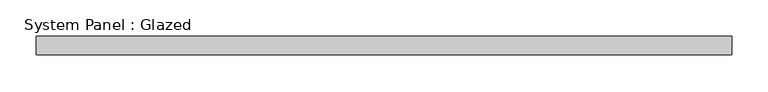
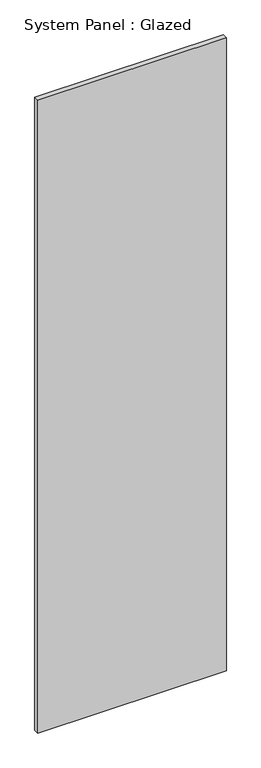
"""IFC4 building model written with IfcOpenShell, lengths in millimetres: plate geometry, System Panel : Glazed."""

from ifc_helpers import new_model, si_unit, origin, origin_with_axes, place, context, project, spatial, polyline, outline, extrude, source, transform, mapped, element, save


def system_panel_glazed_5332cc33(model_context):
    return source(origin(), model_context, "Body", "SweptSolid", [
        extrude(outline(polyline([(476.825, 19.05), (-476.825, 19.05), (-476.825, 44.45), (476.825, 44.45), (476.825, 19.05)])), origin_with_axes(), (0.0, 0.0, 1.0), 3379.9820397),
    ])


if __name__ == "__main__":
    model = new_model("IFC4")
    model_context = context("Model", 3, world=origin())
    ifc_project = project(units=[si_unit("LENGTHUNIT", "METRE", prefix="MILLI")], contexts=[model_context])
    site = spatial("IfcSite", under=ifc_project)
    building = spatial("IfcBuilding", under=site)
    placement = place(None, origin())
    system_panel_glazed_shape = system_panel_glazed_5332cc33(model_context)
    element("IfcPlate", 1, ObjectType="System Panel : Glazed", at=placement, inside=building, context=model_context, shape_type="MappedRepresentation", body=[
        mapped(system_panel_glazed_shape, transform((0.0, 0.0, 0.0), x_axis=(1.0, 0.0, 0.0), y_axis=(0.0, 1.0, 0.0), z_axis=(0.0, 0.0, 1.0))),
    ])
    save(model, "model.ifc")

# Revit data of these elements
# Type "System Panel : Glazed"
#   Construction Type Id = "GSP4R"
#   Analytic Construction = "1/8 in Pilkington single glazing"
#   Visual Light Transmittance = 0.9
#   Solar Heat Gain Coefficient = 0.86
#   Heat Transfer Coefficient (U) = 1.18115 BTU/(h·ft²·°F)
#   Define Thermal Properties by = 1
# Element 1 (IfcPlate, "System Panel : Glazed")
#   Materials on its faces: "Glass"
# Materials
#   "Glass": class "Glass", colour RGB 0 128 192, transparency 0.75, Description = "Soda Lime Glass", Cost = 0
